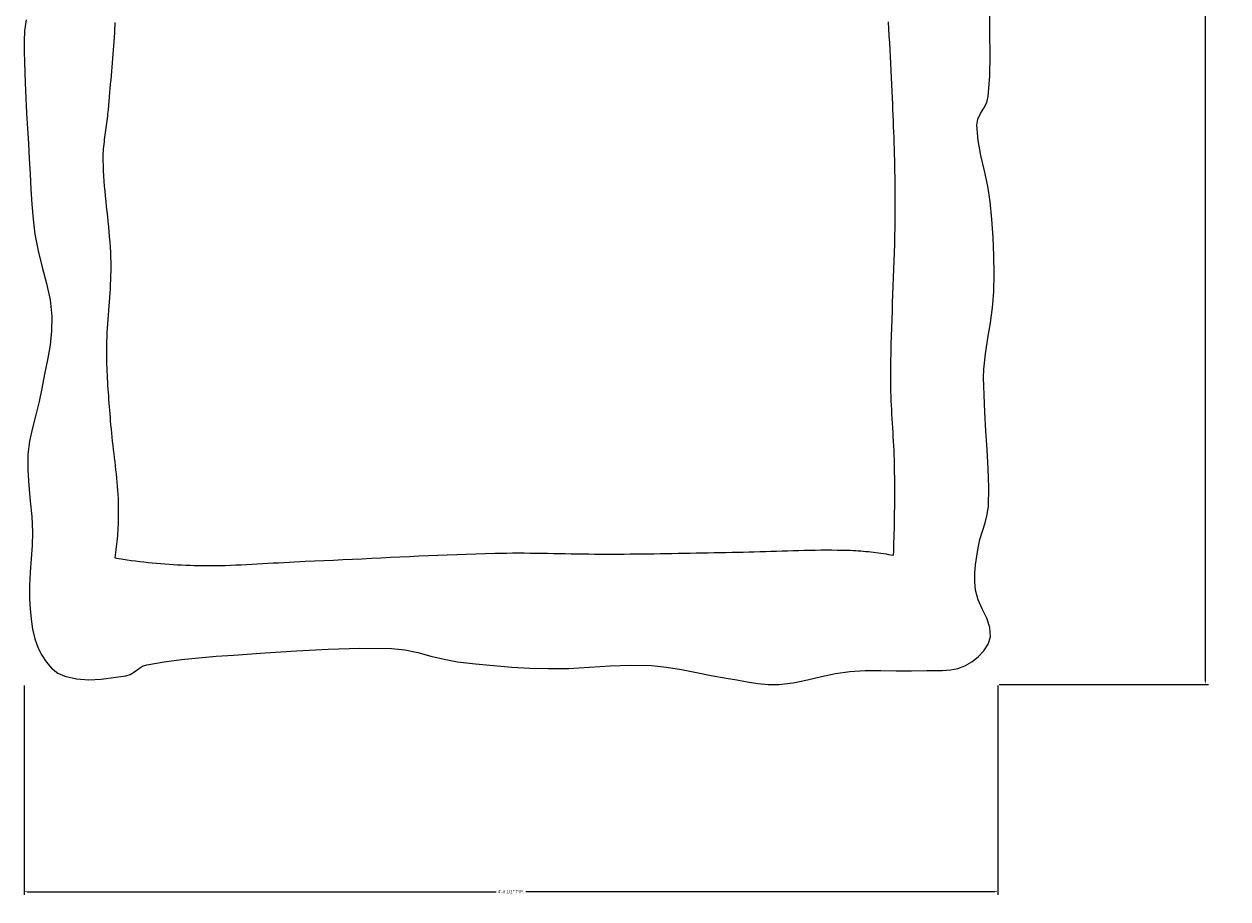
# Model space of a CAD drawing. Units: inches. Extents: x -36302355 to 648, y -221479757 to 75.
# Tile 24 of 37: x 192 to 262, y -268 to -218. Entities that reach past the tile are written whole.
import ezdxf

# ---------------------------------------------------------------- set-up
doc = ezdxf.new("R2010")
doc.units = ezdxf.units.IN
doc.header["$MEASUREMENT"] = 0
doc.layers.add('A-ANNO-DIMS', color=2, linetype='Continuous', lineweight=18)
doc.layers.add('A-FURN', color=8, linetype='Continuous', lineweight=13)
doc.styles.get("Standard").update_dxf_attribs({"font": 'arial.ttf'})
doc.dimstyles.get("Standard").update_dxf_attribs({"dimtxt": 0.18, "dimasz": 0.18, "dimexe": 0.18, "dimexo": 0.0625, "dimgap": 0.09, "dimtad": 0, "dimtih": 1, "dimtoh": 1, "dimdec": 0, "dimzin": 0, "dimdsep": 46, "dimlunit": 3, "dimtxsty": 'Standard', "dimcen": 0.09, "dimadec": 0, "dimazin": 0, "dimtfac": 1, "dimtdec": 0, "dimtofl": 0, "dimtmove": 0, "dimatfit": 3, "dimfxl": 1, "dimtolj": 1, "dimtzin": 0, "dimarcsym": 0})

# ---------------------------------------------------------------- blocks, each defined once
blk = doc.blocks.new('BED-DOUBLE')
for p, q in [((0.112, 38.48), (0.028, 37.836)), ((50.064, 37.953), (50.04, 38.355)), ((55.907, 37.677), (55.898, 38.895)), ((0.028, 37.836), (0, 37.235)), ((5.229, 37.723), (5.213, 37.476)), ((5.244, 37.971), (5.229, 37.723)), ((5.254, 38.144), (5.244, 37.971)), ((5.262, 38.318), (5.254, 38.144)), ((50.087, 37.551), (50.064, 37.953)), ((55.917, 36.459), (55.907, 37.677)), ((0, 37.235), (0, 36.634)), ((5.178, 36.981), (5.159, 36.734)), ((5.196, 37.228), (5.178, 36.981)), ((5.213, 37.476), (5.196, 37.228)), ((50.111, 37.149), (50.087, 37.551)), ((50.134, 36.747), (50.111, 37.149)), ((0, 36.634), (0.018, 36.032)), ((5.12, 36.239), (5.1, 35.992)), ((5.14, 36.487), (5.12, 36.239)), ((5.159, 36.734), (5.14, 36.487)), ((50.157, 36.345), (50.134, 36.747)), ((50.179, 35.943), (50.157, 36.345)), ((55.897, 35.242), (55.917, 36.459)), ((0.018, 36.032), (0.045, 35.43)), ((5.08, 35.745), (5.058, 35.498)), ((5.1, 35.992), (5.08, 35.745)), ((50.201, 35.542), (50.179, 35.943)), ((50.222, 35.14), (50.201, 35.542)), ((0.045, 35.43), (0.071, 34.828)), ((5.015, 35.004), (4.993, 34.757)), ((5.037, 35.251), (5.015, 35.004)), ((5.058, 35.498), (5.037, 35.251)), ((50.241, 34.737), (50.222, 35.14)), ((55.818, 34.029), (55.897, 35.242)), ((0.071, 34.828), (0.107, 33.948)), ((4.949, 34.263), (4.926, 34.016)), ((4.971, 34.51), (4.949, 34.263)), ((4.993, 34.757), (4.971, 34.51)), ((50.259, 34.335), (50.241, 34.737)), ((50.275, 33.933), (50.259, 34.335)), ((0.107, 33.948), (0.149, 33.068)), ((4.882, 33.522), (4.859, 33.275)), ((4.904, 33.769), (4.882, 33.522)), ((4.926, 34.016), (4.904, 33.769)), ((50.287, 33.608), (50.275, 33.933)), ((50.3, 33.282), (50.287, 33.608)), ((55.558, 33.367), (55.726, 33.689)), ((55.726, 33.689), (55.818, 34.029)), ((0.149, 33.068), (0.196, 32.188)), ((4.809, 32.758), (4.793, 32.623)), ((4.824, 32.893), (4.809, 32.758)), ((4.837, 33.028), (4.824, 32.893)), ((4.859, 33.275), (4.837, 33.028)), ((50.312, 32.957), (50.3, 33.282)), ((50.325, 32.632), (50.312, 32.957)), ((55.219, 32.726), (55.37, 33.05)), ((55.37, 33.05), (55.558, 33.367)), ((0.196, 32.188), (0.247, 31.308)), ((4.719, 32.082), (4.7, 31.947)), ((4.739, 32.217), (4.719, 32.082)), ((4.758, 32.352), (4.739, 32.217)), ((4.776, 32.487), (4.758, 32.352)), ((4.793, 32.623), (4.776, 32.487)), ((50.337, 32.306), (50.325, 32.632)), ((50.348, 31.981), (50.337, 32.306)), ((55.16, 32.385), (55.219, 32.726)), ((55.234, 31.495), (55.16, 32.385)), ((4.627, 31.407), (4.612, 31.272)), ((4.644, 31.542), (4.627, 31.407)), ((4.662, 31.677), (4.644, 31.542)), ((4.681, 31.812), (4.662, 31.677)), ((4.7, 31.947), (4.681, 31.812)), ((50.36, 31.655), (50.348, 31.981)), ((50.371, 31.33), (50.36, 31.655)), ((55.394, 30.613), (55.234, 31.495)), ((0.247, 31.308), (0.302, 30.429)), ((4.568, 30.73), (4.563, 30.595)), ((4.576, 30.866), (4.568, 30.73)), ((4.586, 31.001), (4.576, 30.866)), ((4.598, 31.136), (4.586, 31.001)), ((4.612, 31.272), (4.598, 31.136)), ((50.381, 31.004), (50.371, 31.33)), ((50.39, 30.679), (50.381, 31.004)), ((50.399, 30.353), (50.39, 30.679)), ((0.302, 30.429), (0.351, 29.554)), ((4.563, 30.595), (4.561, 30.459)), ((4.561, 30.459), (4.562, 30.323)), ((4.562, 30.323), (4.57, 30.028)), ((4.57, 30.028), (4.583, 29.734)), ((50.408, 30.028), (50.399, 30.353)), ((50.415, 29.702), (50.408, 30.028)), ((55.593, 29.734), (55.394, 30.613)), ((0.351, 29.554), (0.396, 28.679)), ((4.583, 29.734), (4.601, 29.439)), ((4.601, 29.439), (4.621, 29.145)), ((50.421, 29.376), (50.415, 29.702)), ((50.426, 29.051), (50.421, 29.376)), ((55.784, 28.854), (55.593, 29.734)), ((0.396, 28.679), (0.448, 27.804)), ((4.621, 29.145), (4.645, 28.851)), ((4.645, 28.851), (4.671, 28.557)), ((50.43, 28.725), (50.426, 29.051)), ((50.433, 28.4), (50.43, 28.725)), ((55.919, 27.967), (55.784, 28.854)), ((4.671, 28.557), (4.699, 28.263)), ((4.699, 28.263), (4.728, 27.969)), ((4.728, 27.969), (4.759, 27.675)), ((50.435, 28.074), (50.433, 28.4)), ((50.435, 27.749), (50.435, 28.074)), ((56.015, 26.923), (55.919, 27.967)), ((0.448, 27.804), (0.521, 26.932)), ((4.759, 27.675), (4.79, 27.382)), ((4.79, 27.382), (4.821, 27.088)), ((50.429, 26.939), (50.434, 27.423)), ((50.434, 27.423), (50.435, 27.749)), ((0.521, 26.932), (0.625, 26.063)), ((4.821, 27.088), (4.852, 26.794)), ((4.852, 26.794), (4.881, 26.5)), ((4.881, 26.5), (4.909, 26.207)), ((50.422, 26.454), (50.429, 26.939)), ((56.091, 25.876), (56.015, 26.923)), ((0.625, 26.063), (0.809, 25.109)), ((4.909, 26.207), (4.935, 25.913)), ((4.935, 25.913), (4.958, 25.618)), ((50.399, 25.486), (50.412, 25.97)), ((50.412, 25.97), (50.422, 26.454)), ((56.14, 24.828), (56.091, 25.876)), ((0.809, 25.109), (1.05, 24.163)), ((4.958, 25.618), (4.978, 25.324)), ((4.978, 25.324), (4.995, 25.03)), ((50.385, 25.001), (50.399, 25.486)), ((4.995, 25.03), (5.007, 24.735)), ((5.007, 24.735), (5.015, 24.44)), ((5.015, 24.44), (5.018, 24.185)), ((50.353, 24.033), (50.37, 24.517)), ((50.37, 24.517), (50.385, 25.001)), ((56.158, 23.779), (56.14, 24.828)), ((1.05, 24.163), (1.298, 23.22)), ((5.016, 23.931), (5.011, 23.676)), ((5.018, 24.185), (5.016, 23.931)), ((50.336, 23.549), (50.353, 24.033)), ((56.139, 22.73), (56.158, 23.779)), ((1.298, 23.22), (1.501, 22.271)), ((4.991, 23.166), (4.977, 22.912)), ((5.002, 23.421), (4.991, 23.166)), ((5.011, 23.676), (5.002, 23.421)), ((50.299, 22.581), (50.317, 23.065)), ((50.317, 23.065), (50.336, 23.549)), ((4.943, 22.403), (4.924, 22.148)), ((4.961, 22.657), (4.943, 22.403)), ((4.977, 22.912), (4.961, 22.657)), ((50.281, 22.096), (50.299, 22.581)), ((56.069, 21.831), (56.139, 22.73)), ((1.501, 22.271), (1.61, 21.31)), ((4.885, 21.639), (4.866, 21.385)), ((4.905, 21.894), (4.885, 21.639)), ((4.924, 22.148), (4.905, 21.894)), ((50.245, 21.128), (50.263, 21.612)), ((50.263, 21.612), (50.281, 22.096)), ((55.946, 20.936), (56.069, 21.831)), ((1.61, 21.31), (1.596, 20.47)), ((4.847, 21.13), (4.829, 20.876)), ((4.866, 21.385), (4.847, 21.13)), ((50.229, 20.644), (50.245, 21.128)), ((55.8, 20.042), (55.946, 20.936)), ((1.596, 20.47), (1.501, 19.634)), ((4.798, 20.366), (4.785, 20.111)), ((4.812, 20.621), (4.798, 20.366)), ((4.829, 20.876), (4.812, 20.621)), ((50.215, 20.16), (50.229, 20.644)), ((1.501, 19.634), (1.355, 18.801)), ((4.77, 19.602), (4.767, 19.347)), ((4.776, 19.857), (4.77, 19.602)), ((4.785, 20.111), (4.776, 19.857)), ((50.19, 19.191), (50.201, 19.676)), ((50.201, 19.676), (50.215, 20.16)), ((55.663, 19.148), (55.8, 20.042)), ((4.767, 19.347), (4.767, 19.142)), ((4.767, 19.142), (4.77, 18.938)), ((4.77, 18.938), (4.773, 18.733)), ((50.182, 18.707), (50.19, 19.191)), ((55.566, 18.25), (55.663, 19.148)), ((1.355, 18.801), (1.187, 17.969)), ((4.773, 18.733), (4.779, 18.528)), ((4.779, 18.528), (4.786, 18.323)), ((4.786, 18.323), (4.794, 18.119)), ((50.173, 17.738), (50.176, 18.223)), ((50.176, 18.223), (50.182, 18.707)), ((55.546, 17.754), (55.566, 18.25)), ((1.187, 17.969), (1.029, 17.139)), ((4.794, 18.119), (4.803, 17.914)), ((4.803, 17.914), (4.814, 17.71)), ((4.814, 17.71), (4.826, 17.505)), ((4.826, 17.505), (4.838, 17.301)), ((50.174, 17.476), (50.173, 17.738)), ((50.177, 17.214), (50.174, 17.476)), ((55.553, 17.258), (55.546, 17.754)), ((1.029, 17.139), (0.867, 16.371)), ((4.838, 17.301), (4.852, 17.096)), ((4.852, 17.096), (4.866, 16.892)), ((4.866, 16.892), (4.88, 16.688)), ((50.183, 16.952), (50.177, 17.214)), ((50.192, 16.69), (50.183, 16.952)), ((55.576, 16.762), (55.553, 17.258)), ((55.604, 16.266), (55.576, 16.762)), ((0.867, 16.371), (0.673, 15.608)), ((4.88, 16.688), (4.895, 16.483)), ((4.895, 16.483), (4.911, 16.279)), ((4.911, 16.279), (4.927, 16.075)), ((4.927, 16.075), (4.943, 15.87)), ((50.202, 16.429), (50.192, 16.69)), ((50.214, 16.167), (50.202, 16.429)), ((50.227, 15.905), (50.214, 16.167)), ((55.626, 15.769), (55.604, 16.266)), ((0.673, 15.608), (0.479, 14.846)), ((4.943, 15.87), (4.959, 15.666)), ((4.959, 15.666), (4.975, 15.462)), ((4.975, 15.462), (4.991, 15.258)), ((50.241, 15.643), (50.227, 15.905)), ((50.256, 15.381), (50.241, 15.643)), ((50.272, 15.12), (50.256, 15.381)), ((55.678, 14.678), (55.626, 15.769)), ((0.479, 14.846), (0.317, 14.08)), ((4.991, 15.258), (5.01, 15.021)), ((5.01, 15.021), (5.032, 14.784)), ((5.032, 14.784), (5.055, 14.547)), ((50.287, 14.858), (50.272, 15.12)), ((50.303, 14.596), (50.287, 14.858)), ((55.747, 13.587), (55.678, 14.678)), ((0.317, 14.08), (0.222, 13.304)), ((5.055, 14.547), (5.08, 14.31)), ((5.08, 14.31), (5.106, 14.074)), ((5.106, 14.074), (5.133, 13.837)), ((50.319, 14.334), (50.303, 14.596)), ((50.333, 14.073), (50.319, 14.334)), ((50.347, 13.811), (50.333, 14.073)), ((0.222, 13.304), (0.211, 12.406)), ((5.133, 13.837), (5.161, 13.601)), ((5.161, 13.601), (5.189, 13.364)), ((5.189, 13.364), (5.218, 13.128)), ((50.36, 13.549), (50.347, 13.811)), ((50.371, 13.287), (50.36, 13.549)), ((50.381, 13.025), (50.371, 13.287)), ((55.809, 12.496), (55.747, 13.587)), ((5.218, 13.128), (5.246, 12.892)), ((5.246, 12.892), (5.273, 12.655)), ((5.273, 12.655), (5.3, 12.419)), ((50.388, 12.763), (50.381, 13.025)), ((50.394, 12.501), (50.388, 12.763)), ((0.211, 12.406), (0.269, 11.508)), ((5.3, 12.419), (5.325, 12.182)), ((5.325, 12.182), (5.349, 11.946)), ((5.349, 11.946), (5.372, 11.709)), ((50.397, 12.25), (50.394, 12.501)), ((50.4, 11.999), (50.397, 12.25)), ((50.402, 11.747), (50.4, 11.999)), ((55.842, 11.405), (55.809, 12.496)), ((0.269, 11.508), (0.358, 10.61)), ((5.372, 11.709), (5.392, 11.472)), ((5.392, 11.472), (5.41, 11.235)), ((5.41, 11.235), (5.425, 10.998)), ((50.403, 11.496), (50.402, 11.747)), ((50.404, 11.244), (50.403, 11.496)), ((50.404, 10.993), (50.404, 11.244)), ((55.821, 10.315), (55.842, 11.405)), ((0.358, 10.61), (0.444, 9.712)), ((5.425, 10.998), (5.438, 10.76)), ((5.438, 10.76), (5.447, 10.523)), ((5.447, 10.523), (5.452, 10.363)), ((50.4, 10.239), (50.402, 10.49)), ((50.402, 10.49), (50.403, 10.742)), ((50.403, 10.742), (50.404, 10.993)), ((5.452, 10.363), (5.454, 10.202)), ((5.454, 10.202), (5.456, 10.042)), ((5.456, 9.881), (5.454, 9.721)), ((5.456, 10.042), (5.456, 9.881)), ((50.393, 9.736), (50.397, 9.987)), ((50.397, 9.987), (50.4, 10.239)), ((55.631, 9.348), (55.755, 9.827)), ((55.755, 9.827), (55.821, 10.315)), ((0.444, 9.712), (0.487, 8.812)), ((5.432, 9.078), (5.422, 8.918)), ((5.44, 9.239), (5.432, 9.078)), ((5.446, 9.399), (5.44, 9.239)), ((5.451, 9.56), (5.446, 9.399)), ((5.454, 9.721), (5.451, 9.56)), ((50.379, 8.982), (50.384, 9.233)), ((50.384, 9.233), (50.389, 9.485)), ((50.389, 9.485), (50.393, 9.736)), ((55.479, 8.873), (55.631, 9.348)), ((0.487, 8.812), (0.469, 8.039)), ((5.385, 8.437), (5.37, 8.278)), ((5.399, 8.598), (5.385, 8.437)), ((5.412, 8.758), (5.399, 8.598)), ((5.422, 8.918), (5.412, 8.758)), ((50.357, 8.228), (50.365, 8.479)), ((50.365, 8.479), (50.372, 8.731)), ((50.372, 8.731), (50.379, 8.982)), ((55.228, 7.912), (55.334, 8.396)), ((55.334, 8.396), (55.479, 8.873)), ((0.469, 8.039), (0.415, 7.265)), ((5.315, 7.799), (5.293, 7.64)), ((5.335, 7.958), (5.315, 7.799)), ((5.353, 8.118), (5.335, 7.958)), ((5.37, 8.278), (5.353, 8.118)), ((41.63, 7.664), (41.951, 7.672)), ((41.951, 7.672), (42.272, 7.681)), ((42.272, 7.681), (42.593, 7.691)), ((42.593, 7.691), (42.914, 7.701)), ((42.914, 7.701), (43.235, 7.712)), ((43.235, 7.712), (43.556, 7.722)), ((43.556, 7.722), (43.877, 7.732)), ((43.877, 7.732), (44.198, 7.742)), ((44.198, 7.742), (44.519, 7.751)), ((44.519, 7.751), (44.839, 7.76)), ((44.839, 7.76), (45.16, 7.767)), ((45.16, 7.767), (45.481, 7.773)), ((45.481, 7.773), (45.802, 7.778)), ((45.802, 7.778), (46.123, 7.782)), ((46.123, 7.782), (46.444, 7.783)), ((46.444, 7.783), (46.765, 7.783)), ((46.765, 7.783), (47.086, 7.78)), ((47.086, 7.78), (47.407, 7.776)), ((47.407, 7.776), (47.554, 7.772)), ((47.554, 7.772), (47.701, 7.768)), ((47.701, 7.768), (47.847, 7.762)), ((47.847, 7.762), (47.994, 7.755)), ((47.994, 7.755), (48.141, 7.746)), ((48.141, 7.746), (48.288, 7.737)), ((48.288, 7.737), (48.435, 7.726)), ((48.435, 7.726), (48.582, 7.714)), ((48.582, 7.714), (48.728, 7.701)), ((48.728, 7.701), (48.875, 7.686)), ((48.875, 7.686), (49.021, 7.671)), ((49.021, 7.671), (49.167, 7.654)), ((50.33, 7.475), (50.34, 7.726)), ((50.34, 7.726), (50.349, 7.977)), ((50.349, 7.977), (50.357, 8.228)), ((55.153, 7.423), (55.228, 7.912)), ((0.415, 7.265), (0.354, 6.492)), ((5.27, 7.481), (5.246, 7.323)), ((5.246, 7.323), (5.486, 7.284)), ((5.293, 7.64), (5.27, 7.481)), ((5.486, 7.284), (5.727, 7.247)), ((5.727, 7.247), (5.968, 7.212)), ((5.968, 7.212), (6.21, 7.179)), ((6.21, 7.179), (6.451, 7.147)), ((6.451, 7.147), (6.693, 7.117)), ((6.693, 7.117), (6.935, 7.089)), ((6.935, 7.089), (7.178, 7.062)), ((7.178, 7.062), (7.42, 7.038)), ((7.42, 7.038), (7.663, 7.015)), ((7.663, 7.015), (7.906, 6.994)), ((7.906, 6.994), (8.149, 6.974)), ((8.149, 6.974), (8.392, 6.956)), ((13.18, 6.958), (13.488, 6.975)), ((13.488, 6.975), (13.796, 6.993)), ((13.796, 6.993), (14.105, 7.011)), ((14.105, 7.011), (14.413, 7.029)), ((14.413, 7.029), (14.721, 7.047)), ((14.721, 7.047), (15.03, 7.064)), ((15.03, 7.064), (15.338, 7.081)), ((15.338, 7.081), (15.646, 7.097)), ((15.646, 7.097), (15.955, 7.112)), ((15.955, 7.112), (16.263, 7.126)), ((16.263, 7.126), (16.812, 7.149)), ((16.812, 7.149), (17.361, 7.174)), ((17.361, 7.174), (17.911, 7.199)), ((17.911, 7.199), (18.46, 7.225)), ((18.46, 7.225), (19.009, 7.251)), ((19.009, 7.251), (19.558, 7.278)), ((19.558, 7.278), (20.107, 7.305)), ((20.107, 7.305), (20.656, 7.332)), ((20.656, 7.332), (21.206, 7.359)), ((21.206, 7.359), (21.755, 7.385)), ((21.755, 7.385), (22.304, 7.411)), ((22.304, 7.411), (22.853, 7.436)), ((22.853, 7.436), (23.402, 7.461)), ((23.402, 7.461), (23.952, 7.484)), ((23.952, 7.484), (24.501, 7.507)), ((24.501, 7.507), (25.05, 7.528)), ((25.05, 7.528), (25.6, 7.547)), ((25.6, 7.547), (26.149, 7.565)), ((26.149, 7.565), (26.698, 7.581)), ((26.698, 7.581), (27.248, 7.595)), ((27.248, 7.595), (27.588, 7.602)), ((27.588, 7.602), (27.927, 7.606)), ((27.927, 7.606), (28.267, 7.609)), ((28.267, 7.609), (28.607, 7.609)), ((28.607, 7.609), (28.946, 7.608)), ((28.946, 7.608), (29.286, 7.605)), ((29.286, 7.605), (29.626, 7.602)), ((29.626, 7.602), (29.966, 7.597)), ((29.966, 7.597), (30.305, 7.592)), ((30.305, 7.592), (30.645, 7.586)), ((30.645, 7.586), (30.985, 7.579)), ((30.985, 7.579), (31.325, 7.573)), ((31.325, 7.573), (31.664, 7.566)), ((31.664, 7.566), (32.004, 7.56)), ((32.004, 7.56), (32.344, 7.555)), ((32.344, 7.555), (32.684, 7.55)), ((32.684, 7.55), (33.023, 7.546)), ((33.023, 7.546), (33.363, 7.544)), ((33.363, 7.544), (33.703, 7.543)), ((33.703, 7.543), (34.043, 7.543)), ((34.043, 7.543), (34.39, 7.545)), ((34.39, 7.545), (34.737, 7.547)), ((34.737, 7.547), (35.085, 7.55)), ((35.085, 7.55), (35.432, 7.554)), ((35.432, 7.554), (35.779, 7.558)), ((35.779, 7.558), (36.127, 7.563)), ((36.127, 7.563), (36.474, 7.568)), ((36.474, 7.568), (36.821, 7.573)), ((36.821, 7.573), (37.168, 7.579)), ((37.168, 7.579), (37.516, 7.585)), ((37.516, 7.585), (37.863, 7.591)), ((37.863, 7.591), (38.21, 7.598)), ((38.21, 7.598), (38.558, 7.604)), ((38.558, 7.604), (38.905, 7.611)), ((38.905, 7.611), (39.252, 7.618)), ((39.252, 7.618), (39.599, 7.625)), ((39.599, 7.625), (39.947, 7.631)), ((39.947, 7.631), (40.294, 7.638)), ((40.294, 7.638), (40.641, 7.644)), ((40.641, 7.644), (40.989, 7.65)), ((40.989, 7.65), (41.309, 7.657)), ((41.309, 7.657), (41.63, 7.664)), ((49.167, 7.654), (49.313, 7.635)), ((49.313, 7.635), (49.459, 7.616)), ((49.459, 7.616), (49.605, 7.596)), ((49.605, 7.596), (49.75, 7.574)), ((49.75, 7.574), (49.896, 7.551)), ((49.896, 7.551), (50.041, 7.527)), ((50.041, 7.527), (50.185, 7.501)), ((50.185, 7.501), (50.33, 7.475)), ((55.086, 6.932), (55.153, 7.423)), ((0.354, 6.492), (0.312, 5.719)), ((8.392, 6.956), (8.635, 6.941)), ((8.635, 6.941), (8.879, 6.927)), ((8.879, 6.927), (9.122, 6.914)), ((9.122, 6.914), (9.365, 6.904)), ((9.365, 6.904), (9.609, 6.895)), ((9.609, 6.895), (9.852, 6.888)), ((9.852, 6.888), (10.096, 6.883)), ((10.096, 6.883), (10.404, 6.879)), ((10.404, 6.879), (10.713, 6.878)), ((10.713, 6.878), (11.021, 6.88)), ((11.021, 6.88), (11.33, 6.886)), ((11.33, 6.886), (11.638, 6.893)), ((11.638, 6.893), (11.947, 6.903)), ((11.947, 6.903), (12.255, 6.914)), ((12.255, 6.914), (12.563, 6.928)), ((12.563, 6.928), (12.872, 6.942)), ((12.872, 6.942), (13.18, 6.958)), ((55.032, 5.947), (55.042, 6.439)), ((55.042, 6.439), (55.086, 6.932)), ((0.312, 5.719), (0.317, 4.946)), ((55.071, 5.457), (55.032, 5.947)), ((0.317, 4.946), (0.35, 4.366)), ((55.224, 4.905), (55.071, 5.457)), ((55.472, 4.369), (55.224, 4.905)), ((0.35, 4.366), (0.401, 3.783)), ((55.73, 3.838), (55.472, 4.369)), ((0.401, 3.783), (0.486, 3.207)), ((55.915, 3.301), (55.73, 3.838)), ((0.486, 3.207), (0.62, 2.644)), ((55.943, 2.749), (55.915, 3.301)), ((0.62, 2.644), (0.821, 2.105)), ((0.821, 2.105), (1.03, 1.695)), ((55.568, 1.939), (55.814, 2.324)), ((55.814, 2.324), (55.943, 2.749)), ((1.03, 1.695), (1.287, 1.3)), ((8.104, 1.311), (9.104, 1.443)), ((9.104, 1.443), (10.109, 1.546)), ((10.109, 1.546), (11.115, 1.628)), ((11.115, 1.628), (12.122, 1.697)), ((12.122, 1.697), (13.949, 1.822)), ((13.949, 1.822), (15.777, 1.943)), ((15.777, 1.943), (17.605, 2.039)), ((17.605, 2.039), (19.435, 2.09)), ((19.435, 2.09), (21.264, 2.075)), ((21.264, 2.075), (22.035, 1.997)), ((22.035, 1.997), (22.798, 1.838)), ((22.798, 1.838), (23.556, 1.643)), ((23.556, 1.643), (24.315, 1.453)), ((24.315, 1.453), (25.082, 1.315)), ((54.861, 1.307), (55.24, 1.598)), ((55.24, 1.598), (55.568, 1.939)), ((1.287, 1.3), (1.593, 0.945)), ((1.593, 0.945), (1.947, 0.659)), ((6.145, 0.575), (6.384, 0.722)), ((6.384, 0.722), (6.615, 0.893)), ((6.615, 0.893), (6.853, 1.046)), ((6.853, 1.046), (7.11, 1.141)), ((7.11, 1.141), (8.104, 1.311)), ((25.082, 1.315), (26.129, 1.191)), ((26.129, 1.191), (27.178, 1.088)), ((27.178, 1.088), (28.229, 1.007)), ((28.229, 1.007), (29.281, 0.949)), ((29.281, 0.949), (30.334, 0.915)), ((30.334, 0.915), (31.531, 0.929)), ((31.531, 0.929), (32.728, 0.991)), ((32.728, 0.991), (33.925, 1.065)), ((33.925, 1.065), (35.121, 1.111)), ((35.121, 1.111), (36.317, 1.092)), ((36.317, 1.092), (37.189, 1.006)), ((37.189, 1.006), (38.055, 0.862)), ((38.055, 0.862), (38.918, 0.688)), ((46.977, 0.631), (47.803, 0.751)), ((47.803, 0.751), (48.694, 0.802)), ((48.694, 0.802), (49.587, 0.807)), ((49.587, 0.807), (50.481, 0.791)), ((50.481, 0.791), (51.375, 0.779)), ((51.375, 0.779), (52.268, 0.798)), ((52.268, 0.798), (52.717, 0.807)), ((52.717, 0.807), (53.172, 0.809)), ((53.172, 0.809), (53.622, 0.834)), ((53.622, 0.834), (54.056, 0.911)), ((54.056, 0.911), (54.464, 1.069)), ((54.464, 1.069), (54.861, 1.307)), ((1.947, 0.659), (2.35, 0.467)), ((2.35, 0.467), (3.037, 0.316)), ((3.037, 0.316), (3.743, 0.273)), ((3.743, 0.273), (4.46, 0.308)), ((4.46, 0.308), (5.177, 0.39)), ((5.177, 0.39), (5.885, 0.491)), ((5.885, 0.491), (6.145, 0.575)), ((38.918, 0.688), (39.781, 0.511)), ((39.781, 0.511), (40.647, 0.36)), ((40.647, 0.36), (41.254, 0.26)), ((41.254, 0.26), (41.863, 0.152)), ((41.863, 0.152), (42.472, 0.059)), ((42.472, 0.059), (43.083, 0.002)), ((43.083, 0.002), (43.695, 0)), ((43.695, 0), (44.523, 0.095)), ((44.523, 0.095), (45.342, 0.26)), ((45.342, 0.26), (46.158, 0.453)), ((46.158, 0.453), (46.977, 0.631))]:
    blk.add_line(p, q)
blk = doc.blocks.new('*D37')
at = {"layer": 'A-ANNO-DIMS', "color": 0, "lineweight": -2, "transparency": 16777216}
for p, q in [((248.653, -175.809), (260.774, -175.809)), ((260.594, -175.989), (260.594, -215.635)), ((260.594, -255.648), (260.594, -216.001)), ((248.653, -255.828), (260.774, -255.828))]:
    blk.add_line(p, q, dxfattribs=at)
at = {"layer": 'A-ANNO-DIMS', "color": 0, "transparency": 16777216}
for points in [[(260.564, -175.989), (260.624, -175.989), (260.594, -175.809)], [(260.564, -255.648), (260.624, -255.648), (260.594, -255.828)]]:
    blk.add_solid(points, dxfattribs=at)
at = {"layer": 'Defpoints', "color": 0, "transparency": 16777216}
for p in [(248.591, -175.809), (260.594, -175.809), (248.591, -255.828)]:
    blk.add_point(p, dxfattribs=at)
at = {"layer": 'A-ANNO-DIMS', "color": 0, "transparency": 16777216, "insert": (260.594, -215.818), "char_height": 0.18, "attachment_point": 5}
blk.add_mtext('\\A1;DOUBLE BED 6\'-8" TYP.', dxfattribs=at)
blk = doc.blocks.new('*D38')
at = {"layer": 'A-ANNO-DIMS', "color": 0, "lineweight": -2, "transparency": 16777216}
for p, q in [((192.212, -255.89), (192.212, -268.01)), ((248.591, -255.89), (248.591, -268.01)), ((192.392, -267.83), (219.549, -267.83)), ((248.411, -267.83), (221.253, -267.83))]:
    blk.add_line(p, q, dxfattribs=at)
at = {"layer": 'A-ANNO-DIMS', "color": 0, "transparency": 16777216}
for points in [[(192.392, -267.8), (192.392, -267.86), (192.212, -267.83)], [(248.411, -267.8), (248.411, -267.86), (248.591, -267.83)]]:
    blk.add_solid(points, dxfattribs=at)
at = {"layer": 'Defpoints', "color": 0, "transparency": 16777216}
for p in [(192.212, -255.828), (248.591, -255.828), (248.591, -267.83)]:
    blk.add_point(p, dxfattribs=at)
at = {"layer": 'A-ANNO-DIMS', "color": 0, "transparency": 16777216, "insert": (220.401, -267.83), "char_height": 0.18, "attachment_point": 5}
blk.add_mtext('\\A1;4\'-8 1/2" TYP.', dxfattribs=at)

msp = doc.modelspace()

# ---------------------------------------------------------------- block references
at = {"layer": 'A-FURN'}
msp.add_blockref('BED-DOUBLE', (192.212, -255.828), dxfattribs=at)

# ---------------------------------------------------------------- dimensions: what is measured, and where the dimension line sits
at = {"layer": 'A-ANNO-DIMS'}
dim = msp.add_linear_dim(base=(260.594, -175.809), p1=(248.591, -255.828), p2=(248.591, -175.809), angle=90, text='DOUBLE BED <> TYP.', dimstyle='Standard', override={"dimdec": 1, "dimlfac": 1, "dimrnd": 0, "dimzin": 1, "dimdsep": 46, "dimlunit": 4, "dimfrac": 2}, dxfattribs=at)
dim.commit()
dim.dimension.update_dxf_attribs({"geometry": '*D37', "text_midpoint": (260.594, -215.818)})
dim = msp.add_linear_dim(base=(248.591, -267.83), p1=(192.212, -255.828), p2=(248.591, -255.828), text='<> TYP.', dimstyle='Standard', override={"dimdec": 1, "dimlfac": 1, "dimrnd": 0, "dimzin": 1, "dimdsep": 46, "dimlunit": 4, "dimfrac": 2}, dxfattribs=at)
dim.commit()
dim.dimension.update_dxf_attribs({"geometry": '*D38', "text_midpoint": (220.401, -267.83)})

doc.saveas('drawing.dxf')
